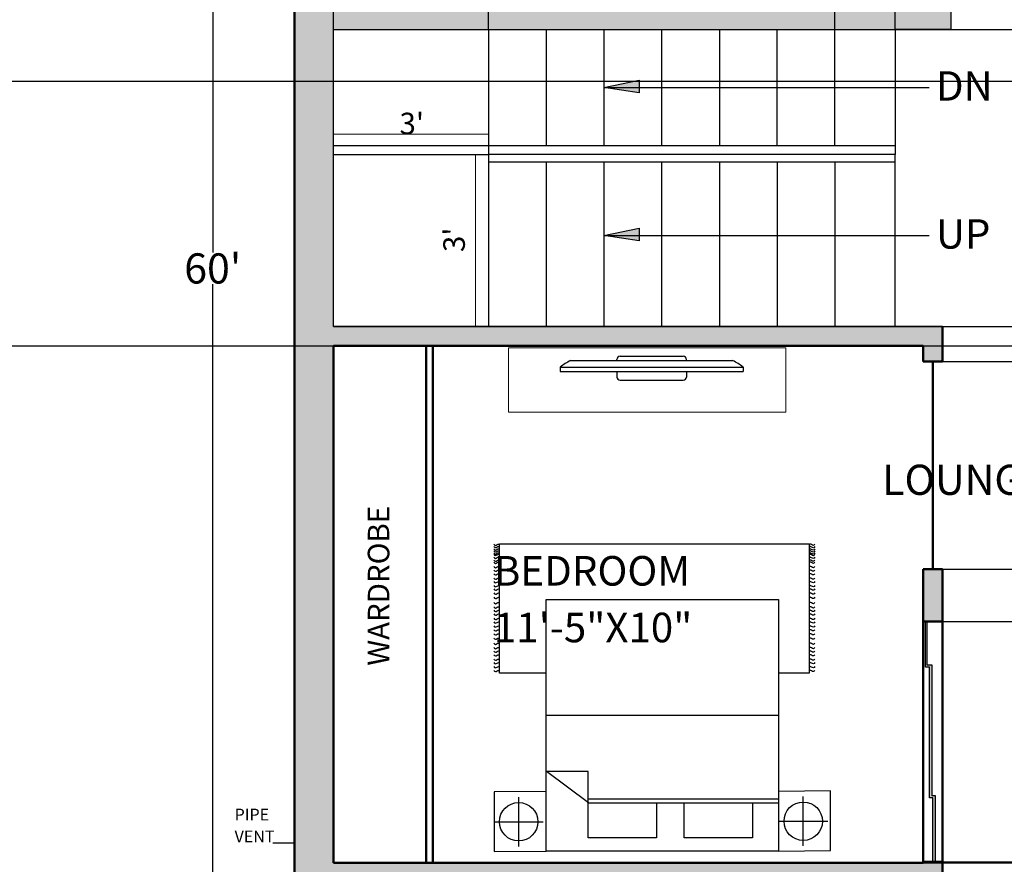
# Model space of a CAD drawing. Units: inches. Extents: x 48 to 822, y -191 to 651.
# Tile 9 of 13: x 445 to 673, y 101 to 297. Entities that reach past the tile are written whole.
import ezdxf

# ---------------------------------------------------------------- set-up
doc = ezdxf.new("R2010")
doc.units = ezdxf.units.IN
doc.header["$MEASUREMENT"] = 0
doc.layers.get('0').update_dxf_attribs({"color": 254})
for name, color, linetype, lineweight in [('A-ANNO-DIMS', 2, 'Continuous', 18), ('A-ANNO-TEXT', 3, 'Continuous', 25), ('A-AREA-IDEN', 7, 'Continuous', 25), ('A-FLOR-STRS', 3, 'Continuous', 25), ('A-FURN', 8, 'Continuous', 18), ('A-GLAZ', 4, 'Continuous', 25), ('A-WALL', 7, 'Continuous', 50), ('A-WALL-PATT', 8, 'Continuous', 13)]:
    doc.layers.add(name, color=color, linetype=linetype, lineweight=lineweight)
doc.layers.add('furniture', color=250, linetype='Continuous')
doc.styles.get("Standard").update_dxf_attribs({"font": 'arial.ttf'})
doc.dimstyles.get("Standard").update_dxf_attribs({"dimtxt": 7, "dimasz": 0.18, "dimexe": 0.18, "dimexo": 0.0625, "dimgap": 0.09, "dimtad": 0, "dimtih": 1, "dimtoh": 1, "dimzin": 0, "dimdsep": 46, "dimlunit": 3, "dimtxsty": 'Standard', "dimcen": 0.09, "dimadec": 0, "dimazin": 0, "dimtfac": 1, "dimtofl": 0, "dimtmove": 0, "dimatfit": 3, "dimfxl": 1, "dimtolj": 1, "dimtzin": 0, "dimarcsym": 0})

# ---------------------------------------------------------------- blocks, each defined once
blk = doc.blocks.new('CARPET')
at = {"layer": 'furniture'}
for p, q in [((-51.53, -98.11), (-51.53, -55.12)), ((-51.53, -55.12), (-41.27, -55.12)), ((36, -55.12), (51.55, -55.12)), ((51.55, -55.12), (51.55, -98.11)), ((51.55, -98.11), (-51.53, -98.11))]:
    blk.add_line(p, q, dxfattribs=at)
for points, knots in [([(-53.37, -55.99), (-53.22, -55.8), (-52.9, -55.41), (-52.34, -55.8), (-51.89, -56.08), (-51.65, -55.91), (-51.53, -55.83)], [0, 0, 0, 0, 0.653278, 1.290138, 1.740457, 2.114451, 2.114451, 2.114451, 2.114451]), ([(53.37, -55.99), (53.22, -55.8), (52.9, -55.41), (52.34, -55.8), (51.89, -56.08), (51.65, -55.91), (51.53, -55.83)], [0, 0, 0, 0, 0.653278, 1.290138, 1.740457, 2.114451, 2.114451, 2.114451, 2.114451]), ([(-53.37, -57.26), (-53.22, -57.07), (-52.9, -56.67), (-52.34, -57.07), (-51.89, -57.35), (-51.65, -57.17), (-51.53, -57.1)], [0, 0, 0, 0, 0.653278, 1.290138, 1.740457, 2.114451, 2.114451, 2.114451, 2.114451]), ([(-53.37, -58.59), (-53.22, -58.4), (-52.9, -58.01), (-52.34, -58.4), (-51.89, -58.68), (-51.65, -58.5), (-51.53, -58.43)], [0, 0, 0, 0, 0.653278, 1.290138, 1.740457, 2.114451, 2.114451, 2.114451, 2.114451]), ([(53.37, -57.26), (53.22, -57.07), (52.9, -56.67), (52.34, -57.07), (51.89, -57.35), (51.65, -57.17), (51.53, -57.1)], [0, 0, 0, 0, 0.653278, 1.290138, 1.740457, 2.114451, 2.114451, 2.114451, 2.114451]), ([(53.37, -58.59), (53.22, -58.4), (52.9, -58.01), (52.34, -58.4), (51.89, -58.68), (51.65, -58.5), (51.53, -58.43)], [0, 0, 0, 0, 0.653278, 1.290138, 1.740457, 2.114451, 2.114451, 2.114451, 2.114451]), ([(-53.37, -59.78), (-53.22, -59.58), (-52.9, -59.19), (-52.34, -59.58), (-51.89, -59.86), (-51.65, -59.69), (-51.53, -59.61)], [0, 0, 0, 0, 0.653278, 1.290138, 1.740457, 2.114451, 2.114451, 2.114451, 2.114451]), ([(-53.37, -61.22), (-53.22, -61.02), (-52.9, -60.63), (-52.34, -61.02), (-51.89, -61.3), (-51.65, -61.13), (-51.53, -61.05)], [0, 0, 0, 0, 0.653278, 1.290138, 1.740457, 2.114451, 2.114451, 2.114451, 2.114451]), ([(-53.37, -62.44), (-53.22, -62.25), (-52.9, -61.86), (-52.34, -62.25), (-51.89, -62.53), (-51.65, -62.36), (-51.53, -62.28)], [0, 0, 0, 0, 0.653278, 1.290138, 1.740457, 2.114451, 2.114451, 2.114451, 2.114451]), ([(53.37, -59.78), (53.22, -59.58), (52.9, -59.19), (52.34, -59.58), (51.89, -59.86), (51.65, -59.69), (51.53, -59.61)], [0, 0, 0, 0, 0.653278, 1.290138, 1.740457, 2.114451, 2.114451, 2.114451, 2.114451]), ([(53.37, -61.22), (53.22, -61.02), (52.9, -60.63), (52.34, -61.02), (51.89, -61.3), (51.65, -61.13), (51.53, -61.05)], [0, 0, 0, 0, 0.653278, 1.290138, 1.740457, 2.114451, 2.114451, 2.114451, 2.114451]), ([(53.37, -62.44), (53.22, -62.25), (52.9, -61.86), (52.34, -62.25), (51.89, -62.53), (51.65, -62.36), (51.53, -62.28)], [0, 0, 0, 0, 0.653278, 1.290138, 1.740457, 2.114451, 2.114451, 2.114451, 2.114451]), ([(-53.37, -63.63), (-53.22, -63.43), (-52.9, -63.04), (-52.34, -63.43), (-51.89, -63.72), (-51.65, -63.54), (-51.53, -63.46)], [0, 0, 0, 0, 0.653278, 1.290138, 1.740457, 2.114451, 2.114451, 2.114451, 2.114451]), ([(-53.37, -65.07), (-53.22, -64.87), (-52.9, -64.48), (-52.34, -64.87), (-51.89, -65.15), (-51.65, -64.98), (-51.53, -64.9)], [0, 0, 0, 0, 0.653278, 1.290138, 1.740457, 2.114451, 2.114451, 2.114451, 2.114451]), ([(53.37, -63.63), (53.22, -63.43), (52.9, -63.04), (52.34, -63.43), (51.89, -63.72), (51.65, -63.54), (51.53, -63.46)], [0, 0, 0, 0, 0.653278, 1.290138, 1.740457, 2.114451, 2.114451, 2.114451, 2.114451]), ([(53.37, -65.07), (53.22, -64.87), (52.9, -64.48), (52.34, -64.87), (51.89, -65.15), (51.65, -64.98), (51.53, -64.9)], [0, 0, 0, 0, 0.653278, 1.290138, 1.740457, 2.114451, 2.114451, 2.114451, 2.114451]), ([(-53.37, -66.76), (-53.22, -66.56), (-52.9, -66.17), (-52.34, -66.56), (-51.89, -66.84), (-51.65, -66.67), (-51.53, -66.59)], [0, 0, 0, 0, 0.653278, 1.290138, 1.740457, 2.114451, 2.114451, 2.114451, 2.114451]), ([(-53.37, -68.2), (-53.22, -68), (-52.9, -67.61), (-52.34, -68), (-51.89, -68.28), (-51.65, -68.11), (-51.53, -68.03)], [0, 0, 0, 0, 0.653278, 1.290138, 1.740457, 2.114451, 2.114451, 2.114451, 2.114451]), ([(53.37, -66.76), (53.22, -66.56), (52.9, -66.17), (52.34, -66.56), (51.89, -66.84), (51.65, -66.67), (51.53, -66.59)], [0, 0, 0, 0, 0.653278, 1.290138, 1.740457, 2.114451, 2.114451, 2.114451, 2.114451]), ([(53.37, -68.2), (53.22, -68), (52.9, -67.61), (52.34, -68), (51.89, -68.28), (51.65, -68.11), (51.53, -68.03)], [0, 0, 0, 0, 0.653278, 1.290138, 1.740457, 2.114451, 2.114451, 2.114451, 2.114451]), ([(-53.37, -69.53), (-53.22, -69.33), (-52.9, -68.94), (-52.34, -69.33), (-51.89, -69.61), (-51.65, -69.44), (-51.53, -69.36)], [0, 0, 0, 0, 0.653278, 1.290138, 1.740457, 2.114451, 2.114451, 2.114451, 2.114451]), ([(-53.37, -70.79), (-53.22, -70.6), (-52.9, -70.21), (-52.34, -70.6), (-51.89, -70.88), (-51.65, -70.7), (-51.53, -70.63)], [0, 0, 0, 0, 0.653278, 1.290138, 1.740457, 2.114451, 2.114451, 2.114451, 2.114451]), ([(-53.37, -72.12), (-53.22, -71.93), (-52.9, -71.54), (-52.34, -71.93), (-51.89, -72.21), (-51.65, -72.04), (-51.53, -71.96)], [0, 0, 0, 0, 0.653278, 1.290138, 1.740457, 2.114451, 2.114451, 2.114451, 2.114451]), ([(53.37, -69.53), (53.22, -69.33), (52.9, -68.94), (52.34, -69.33), (51.89, -69.61), (51.65, -69.44), (51.53, -69.36)], [0, 0, 0, 0, 0.653278, 1.290138, 1.740457, 2.114451, 2.114451, 2.114451, 2.114451]), ([(53.37, -70.79), (53.22, -70.6), (52.9, -70.21), (52.34, -70.6), (51.89, -70.88), (51.65, -70.7), (51.53, -70.63)], [0, 0, 0, 0, 0.653278, 1.290138, 1.740457, 2.114451, 2.114451, 2.114451, 2.114451]), ([(53.37, -72.12), (53.22, -71.93), (52.9, -71.54), (52.34, -71.93), (51.89, -72.21), (51.65, -72.04), (51.53, -71.96)], [0, 0, 0, 0, 0.653278, 1.290138, 1.740457, 2.114451, 2.114451, 2.114451, 2.114451]), ([(-53.37, -73.31), (-53.22, -73.11), (-52.9, -72.72), (-52.34, -73.11), (-51.89, -73.4), (-51.65, -73.22), (-51.53, -73.14)], [0, 0, 0, 0, 0.653278, 1.290138, 1.740457, 2.114451, 2.114451, 2.114451, 2.114451]), ([(-53.37, -74.75), (-53.22, -74.55), (-52.9, -74.16), (-52.34, -74.55), (-51.89, -74.83), (-51.65, -74.66), (-51.53, -74.58)], [0, 0, 0, 0, 0.653278, 1.290138, 1.740457, 2.114451, 2.114451, 2.114451, 2.114451]), ([(53.37, -73.31), (53.22, -73.11), (52.9, -72.72), (52.34, -73.11), (51.89, -73.4), (51.65, -73.22), (51.53, -73.14)], [0, 0, 0, 0, 0.653278, 1.290138, 1.740457, 2.114451, 2.114451, 2.114451, 2.114451]), ([(53.37, -74.75), (53.22, -74.55), (52.9, -74.16), (52.34, -74.55), (51.89, -74.83), (51.65, -74.66), (51.53, -74.58)], [0, 0, 0, 0, 0.653278, 1.290138, 1.740457, 2.114451, 2.114451, 2.114451, 2.114451]), ([(-53.37, -75.98), (-53.22, -75.78), (-52.9, -75.39), (-52.34, -75.78), (-51.89, -76.06), (-51.65, -75.89), (-51.53, -75.81)], [0, 0, 0, 0, 0.653278, 1.290138, 1.740457, 2.114451, 2.114451, 2.114451, 2.114451]), ([(-53.37, -77.16), (-53.22, -76.96), (-52.9, -76.57), (-52.34, -76.96), (-51.89, -77.25), (-51.65, -77.07), (-51.53, -76.99)], [0, 0, 0, 0, 0.653278, 1.290138, 1.740457, 2.114451, 2.114451, 2.114451, 2.114451]), ([(-53.37, -78.6), (-53.22, -78.4), (-52.9, -78.01), (-52.34, -78.4), (-51.89, -78.68), (-51.65, -78.51), (-51.53, -78.43)], [0, 0, 0, 0, 0.653278, 1.290138, 1.740457, 2.114451, 2.114451, 2.114451, 2.114451]), ([(53.37, -75.98), (53.22, -75.78), (52.9, -75.39), (52.34, -75.78), (51.89, -76.06), (51.65, -75.89), (51.53, -75.81)], [0, 0, 0, 0, 0.653278, 1.290138, 1.740457, 2.114451, 2.114451, 2.114451, 2.114451]), ([(53.37, -77.16), (53.22, -76.96), (52.9, -76.57), (52.34, -76.96), (51.89, -77.25), (51.65, -77.07), (51.53, -76.99)], [0, 0, 0, 0, 0.653278, 1.290138, 1.740457, 2.114451, 2.114451, 2.114451, 2.114451]), ([(53.37, -78.6), (53.22, -78.4), (52.9, -78.01), (52.34, -78.4), (51.89, -78.68), (51.65, -78.51), (51.53, -78.43)], [0, 0, 0, 0, 0.653278, 1.290138, 1.740457, 2.114451, 2.114451, 2.114451, 2.114451]), ([(-53.37, -80.29), (-53.22, -80.09), (-52.9, -79.7), (-52.34, -80.09), (-51.89, -80.37), (-51.65, -80.2), (-51.53, -80.12)], [0, 0, 0, 0, 0.653278, 1.290138, 1.740457, 2.114451, 2.114451, 2.114451, 2.114451]), ([(-53.37, -81.73), (-53.22, -81.53), (-52.9, -81.14), (-52.34, -81.53), (-51.89, -81.81), (-51.65, -81.64), (-51.53, -81.56)], [0, 0, 0, 0, 0.653278, 1.290138, 1.740457, 2.114451, 2.114451, 2.114451, 2.114451]), ([(53.37, -80.29), (53.22, -80.09), (52.9, -79.7), (52.34, -80.09), (51.89, -80.37), (51.65, -80.2), (51.53, -80.12)], [0, 0, 0, 0, 0.653278, 1.290138, 1.740457, 2.114451, 2.114451, 2.114451, 2.114451]), ([(53.37, -81.73), (53.22, -81.53), (52.9, -81.14), (52.34, -81.53), (51.89, -81.81), (51.65, -81.64), (51.53, -81.56)], [0, 0, 0, 0, 0.653278, 1.290138, 1.740457, 2.114451, 2.114451, 2.114451, 2.114451]), ([(-53.37, -83.06), (-53.22, -82.86), (-52.9, -82.47), (-52.34, -82.86), (-51.89, -83.14), (-51.65, -82.97), (-51.53, -82.89)], [0, 0, 0, 0, 0.653278, 1.290138, 1.740457, 2.114451, 2.114451, 2.114451, 2.114451]), ([(-53.37, -84.18), (-53.22, -83.99), (-52.9, -83.6), (-52.34, -83.99), (-51.89, -84.27), (-51.65, -84.09), (-51.53, -84.02)], [0, 0, 0, 0, 0.653278, 1.290138, 1.740457, 2.114451, 2.114451, 2.114451, 2.114451]), ([(-53.37, -85.51), (-53.22, -85.32), (-52.9, -84.93), (-52.34, -85.32), (-51.89, -85.6), (-51.65, -85.42), (-51.53, -85.35)], [0, 0, 0, 0, 0.653278, 1.290138, 1.740457, 2.114451, 2.114451, 2.114451, 2.114451]), ([(53.37, -83.06), (53.22, -82.86), (52.9, -82.47), (52.34, -82.86), (51.89, -83.14), (51.65, -82.97), (51.53, -82.89)], [0, 0, 0, 0, 0.653278, 1.290138, 1.740457, 2.114451, 2.114451, 2.114451, 2.114451]), ([(53.37, -84.18), (53.22, -83.99), (52.9, -83.6), (52.34, -83.99), (51.89, -84.27), (51.65, -84.09), (51.53, -84.02)], [0, 0, 0, 0, 0.653278, 1.290138, 1.740457, 2.114451, 2.114451, 2.114451, 2.114451]), ([(53.37, -85.51), (53.22, -85.32), (52.9, -84.93), (52.34, -85.32), (51.89, -85.6), (51.65, -85.42), (51.53, -85.35)], [0, 0, 0, 0, 0.653278, 1.290138, 1.740457, 2.114451, 2.114451, 2.114451, 2.114451]), ([(-53.37, -86.7), (-53.22, -86.5), (-52.9, -86.11), (-52.34, -86.5), (-51.89, -86.78), (-51.65, -86.61), (-51.53, -86.53)], [0, 0, 0, 0, 0.653278, 1.290138, 1.740457, 2.114451, 2.114451, 2.114451, 2.114451]), ([(-53.37, -88.14), (-53.22, -87.94), (-52.9, -87.55), (-52.34, -87.94), (-51.89, -88.22), (-51.65, -88.05), (-51.53, -87.97)], [0, 0, 0, 0, 0.653278, 1.290138, 1.740457, 2.114451, 2.114451, 2.114451, 2.114451]), ([(53.37, -86.7), (53.22, -86.5), (52.9, -86.11), (52.34, -86.5), (51.89, -86.78), (51.65, -86.61), (51.53, -86.53)], [0, 0, 0, 0, 0.653278, 1.290138, 1.740457, 2.114451, 2.114451, 2.114451, 2.114451]), ([(53.37, -88.14), (53.22, -87.94), (52.9, -87.55), (52.34, -87.94), (51.89, -88.22), (51.65, -88.05), (51.53, -87.97)], [0, 0, 0, 0, 0.653278, 1.290138, 1.740457, 2.114451, 2.114451, 2.114451, 2.114451]), ([(-53.37, -89.36), (-53.22, -89.17), (-52.9, -88.78), (-52.34, -89.17), (-51.89, -89.45), (-51.65, -89.28), (-51.53, -89.2)], [0, 0, 0, 0, 0.653278, 1.290138, 1.740457, 2.114451, 2.114451, 2.114451, 2.114451]), ([(-53.37, -90.55), (-53.22, -90.35), (-52.9, -89.96), (-52.34, -90.35), (-51.89, -90.64), (-51.65, -90.46), (-51.53, -90.38)], [0, 0, 0, 0, 0.653278, 1.290138, 1.740457, 2.114451, 2.114451, 2.114451, 2.114451]), ([(-53.37, -91.99), (-53.22, -91.79), (-52.9, -91.4), (-52.34, -91.79), (-51.89, -92.07), (-51.65, -91.9), (-51.53, -91.82)], [0, 0, 0, 0, 0.653278, 1.290138, 1.740457, 2.114451, 2.114451, 2.114451, 2.114451]), ([(53.37, -89.36), (53.22, -89.17), (52.9, -88.78), (52.34, -89.17), (51.89, -89.45), (51.65, -89.28), (51.53, -89.2)], [0, 0, 0, 0, 0.653278, 1.290138, 1.740457, 2.114451, 2.114451, 2.114451, 2.114451]), ([(53.37, -90.55), (53.22, -90.35), (52.9, -89.96), (52.34, -90.35), (51.9, -90.63), (51.66, -90.47), (51.55, -90.4)], [0, 0, 0, 0, 0.653278, 1.290138, 1.740457, 2.0926, 2.0926, 2.0926, 2.0926]), ([(53.37, -91.99), (53.22, -91.79), (52.9, -91.4), (52.34, -91.79), (51.9, -92.07), (51.66, -91.91), (51.55, -91.83)], [0, 0, 0, 0, 0.653278, 1.290138, 1.740457, 2.0926, 2.0926, 2.0926, 2.0926]), ([(-53.37, -92.69), (-53.22, -92.48), (-52.9, -92.08), (-52.35, -92.49), (-51.89, -92.77), (-51.65, -92.6), (-51.53, -92.52)], [0, 0, 0, 0, 0.663904, 1.307406, 1.757725, 2.131719, 2.131719, 2.131719, 2.131719]), ([(-53.37, -93.61), (-53.22, -93.42), (-52.9, -93.03), (-52.34, -93.42), (-51.89, -93.7), (-51.65, -93.52), (-51.53, -93.45)], [0, 0, 0, 0, 0.653278, 1.290138, 1.740457, 2.114451, 2.114451, 2.114451, 2.114451]), ([(-53.37, -94.55), (-53.22, -94.35), (-52.9, -93.96), (-52.34, -94.35), (-51.89, -94.63), (-51.65, -94.46), (-51.53, -94.38)], [0, 0, 0, 0, 0.653278, 1.290138, 1.740457, 2.114451, 2.114451, 2.114451, 2.114451]), ([(-53.37, -95.05), (-53.22, -94.85), (-52.9, -94.46), (-52.34, -94.85), (-51.89, -95.14), (-51.65, -94.96), (-51.53, -94.88)], [0, 0, 0, 0, 0.653278, 1.290138, 1.740457, 2.114451, 2.114451, 2.114451, 2.114451]), ([(53.37, -92.69), (53.22, -92.49), (52.9, -92.09), (52.34, -92.49), (51.9, -92.77), (51.66, -92.61), (51.55, -92.53)], [0, 0, 0, 0, 0.656792, 1.295826, 1.746145, 2.098292, 2.098292, 2.098292, 2.098292]), ([(53.37, -93.66), (53.22, -93.46), (52.9, -93.07), (52.34, -93.46), (51.9, -93.74), (51.66, -93.58), (51.55, -93.5)], [0, 0, 0, 0, 0.653278, 1.290138, 1.740457, 2.0926, 2.0926, 2.0926, 2.0926]), ([(53.37, -94.59), (53.22, -94.4), (52.9, -94.01), (52.34, -94.4), (51.9, -94.68), (51.66, -94.51), (51.55, -94.44)], [0, 0, 0, 0, 0.653278, 1.290138, 1.740457, 2.0926, 2.0926, 2.0926, 2.0926]), ([(53.37, -95.1), (53.22, -94.9), (52.9, -94.51), (52.34, -94.9), (51.9, -95.18), (51.66, -95.02), (51.55, -94.94)], [0, 0, 0, 0, 0.653278, 1.290138, 1.740457, 2.0926, 2.0926, 2.0926, 2.0926]), ([(-53.37, -95.73), (-53.22, -95.54), (-52.9, -95.15), (-52.34, -95.54), (-51.89, -95.82), (-51.65, -95.65), (-51.53, -95.57)], [0, 0, 0, 0, 0.653278, 1.290138, 1.740457, 2.114451, 2.114451, 2.114451, 2.114451]), ([(-53.37, -96.38), (-53.22, -96.18), (-52.9, -95.79), (-52.34, -96.18), (-51.89, -96.47), (-51.65, -96.29), (-51.53, -96.21)], [0, 0, 0, 0, 0.653278, 1.290138, 1.740457, 2.114451, 2.114451, 2.114451, 2.114451]), ([(-53.37, -97.17), (-53.22, -96.98), (-52.9, -96.59), (-52.34, -96.98), (-51.89, -97.26), (-51.65, -97.08), (-51.53, -97.01)], [0, 0, 0, 0, 0.653278, 1.290138, 1.740457, 2.114451, 2.114451, 2.114451, 2.114451]), ([(-53.37, -97.99), (-53.22, -97.79), (-52.9, -97.4), (-52.34, -97.79), (-51.89, -98.08), (-51.65, -97.9), (-51.53, -97.82)], [0, 0, 0, 0, 0.653278, 1.290138, 1.740457, 2.114451, 2.114451, 2.114451, 2.114451]), ([(53.37, -95.78), (53.22, -95.58), (52.9, -95.19), (52.34, -95.58), (51.89, -95.86), (51.65, -95.69), (51.53, -95.61)], [0, 0, 0, 0, 0.653278, 1.290138, 1.740457, 2.114451, 2.114451, 2.114451, 2.114451]), ([(53.37, -96.43), (53.22, -96.23), (52.9, -95.84), (52.34, -96.23), (51.89, -96.51), (51.65, -96.34), (51.53, -96.26)], [0, 0, 0, 0, 0.653278, 1.290138, 1.740457, 2.114451, 2.114451, 2.114451, 2.114451]), ([(53.37, -97.22), (53.22, -97.02), (52.9, -96.63), (52.34, -97.02), (51.89, -97.3), (51.65, -97.13), (51.53, -97.05)], [0, 0, 0, 0, 0.653278, 1.290138, 1.740457, 2.114451, 2.114451, 2.114451, 2.114451]), ([(53.37, -97.99), (53.22, -97.79), (52.9, -97.4), (52.34, -97.79), (51.89, -98.08), (51.65, -97.9), (51.53, -97.82)], [0, 0, 0, 0, 0.653278, 1.290138, 1.740457, 2.114451, 2.114451, 2.114451, 2.114451])]:
    blk.add_open_spline(points, degree=3, knots=knots, dxfattribs=at)
blk = doc.blocks.new('A$C58D270C6')
at = {"layer": 'furniture'}
for p, q in [((9.09, 124.13), (9.09, 108.87)), ((1.46, 116.5), (16.73, 116.5)), ((14.97, 94.84), (24.62, 107.92)), ((24.62, 94.93), (24.62, 107.92)), ((42.08, 108), (42.08, 36)), ((14.97, 94.93), (24.62, 94.93)), ((14.97, 94.84), (14.97, 36)), ((16.22, 94.93), (16.22, 36)), ((9.25, 36), (9.25, 20.74)), ((1.62, 28.37), (16.88, 28.37))]:
    blk.add_line(p, q, dxfattribs=at)
for points in [[(18.5, 108), (18.34, 124.13), (-0.16, 124.13), (0, 108)], [(0, 108), (77.91, 108), (77.91, 36), (0, 36)], [(4.09, 94.93), (14.97, 94.93), (14.97, 73.83), (4.09, 73.83)], [(4.09, 65.23), (14.97, 65.23), (14.97, 44.13), (4.09, 44.13)], [(18.65, 19.87), (18.5, 36), (0, 36), (0.16, 19.87)]]:
    blk.add_lwpolyline(points, close=True, dxfattribs=at)
for centre in [(9.09, 116.5), (9.25, 28.37)]:
    blk.add_circle(centre, 5.95, dxfattribs=at)
at = {"layer": 'furniture', "xscale": 0.9312884925094044, "yscale": 0.9312884925094044, "zscale": 0.9312884925094044, "rotation": 90}
blk.add_blockref('CARPET', (3.79, 74.47), dxfattribs=at)
blk = doc.blocks.new('PLASMA-LARGE')
at = {"layer": 'furniture'}
for p, q in [((-7.26, 0), (7.26, 0)), ((-18.61, -1), (18.61, -1)), ((-8, -1), (-8, -0.74)), ((8, -1), (8, -0.74)), ((-21, -2.5), (21, -2.5)), ((-21, -2.5), (-21, -3.5)), ((-21, -3.5), (21, -3.5)), ((-8, -3.5), (-8, -4.76)), ((8, -3.5), (8, -4.76)), ((21, -2.5), (21, -3.5)), ((-7.26, -5.5), (7.26, -5.5))]:
    blk.add_line(p, q, dxfattribs=at)
for centre, radius, start, end in [((-7.26, -0.74), 0.744, 90, 180), ((7.26, -0.74), 0.744, 0, 90), ((-13.97, -11.05), 11.07, 114.7602, 129.4175), ((13.97, -11.05), 11.07, 50.5825, 65.2398), ((-7.26, -4.76), 0.744, 180, 270), ((7.26, -4.76), 0.744, 270, 0)]:
    blk.add_arc(centre, radius, start, end, dxfattribs=at)
blk = doc.blocks.new('*D19')
at = {"layer": 'A-ANNO-DIMS', "color": 0, "lineweight": -2, "transparency": 16777216}
for p, q in [((489.56, 599.69), (489.41, 599.69)), ((489.59, 599.51), (489.59, 243.35)), ((489.59, -120.13), (489.59, 236.02)), ((489.56, -120.31), (489.41, -120.31))]:
    blk.add_line(p, q, dxfattribs=at)
at = {"layer": 'A-ANNO-DIMS', "color": 0, "transparency": 16777216}
for points in [[(489.56, 599.51), (489.62, 599.51), (489.59, 599.69)], [(489.56, -120.13), (489.62, -120.13), (489.59, -120.31)]]:
    blk.add_solid(points, dxfattribs=at)
at = {"layer": 'Defpoints', "color": 0, "transparency": 16777216}
for p in [(489.62, 599.69), (489.59, -120.31), (489.62, -120.31)]:
    blk.add_point(p, dxfattribs=at)
at = {"layer": 'A-ANNO-DIMS', "color": 0, "transparency": 16777216, "insert": (489.59, 239.69), "char_height": 7, "attachment_point": 5}
blk.add_mtext("\\A1;60'", dxfattribs=at)
blk = doc.blocks.new('WIN-1500')
for p, q in [((315.51, 546.44), (315.51, 547.24)), ((315.51, 547.24), (345.84, 547.24)), ((345.84, 547.24), (345.84, 548.17)), ((345.84, 548.17), (356.45, 548.17)), ((346.31, 546.59), (346.31, 547.73)), ((346.31, 547.73), (356.45, 547.73)), ((300.62, 546.44), (315.51, 546.44)), ((300.62, 545.8), (315.95, 545.8)), ((315.95, 545.8), (315.95, 546.59)), ((315.95, 546.59), (346.31, 546.59))]:
    blk.add_line(p, q)
blk = doc.blocks.new('TV-UNIT')
for p, q in [((14.9, 64.44), (0, 64.44)), ((0, 64.44), (0, 0)), ((14.9, 64.44), (14.9, 0)), ((0, 0), (14.9, 0))]:
    blk.add_line(p, q)
blk = doc.blocks.new('STAIR-ARROW')
for p, q in [((0, 1.28), (8.17, 2.92)), ((8.17, 2.92), (8.17, 0)), ((0, 1.28), (75.57, 1.28)), ((8.17, 0), (0, 1.28))]:
    blk.add_line(p, q)
blk = doc.blocks.new('*D52')
at = {"layer": 'A-ANNO-DIMS', "color": 0, "lineweight": -2, "transparency": 16777216}
for p, q in [((713, 201.45), (709.64, 201.45)), ((709.82, 201.27), (709.82, 194.33)), ((709.82, 179.96), (709.82, 186.9)), ((713, 179.78), (709.64, 179.78))]:
    blk.add_line(p, q, dxfattribs=at)
at = {"layer": 'A-ANNO-DIMS', "color": 0, "transparency": 16777216}
for points in [[(709.79, 201.27), (709.85, 201.27), (709.82, 201.45)], [(709.79, 179.96), (709.85, 179.96), (709.82, 179.78)]]:
    blk.add_solid(points, dxfattribs=at)
at = {"layer": 'Defpoints', "color": 0, "transparency": 16777216}
for p in [(709.82, 201.45), (713.07, 201.45), (713.07, 179.78)]:
    blk.add_point(p, dxfattribs=at)
at = {"layer": 'A-ANNO-DIMS', "color": 0, "transparency": 16777216, "insert": (709.82, 190.62), "char_height": 7, "attachment_point": 5}
blk.add_mtext('\\A1;LOUNGE CHAIR 1\'-9 1/2" TYP.', dxfattribs=at)
blk = doc.blocks.new('*D85')
at = {"layer": 'A-ANNO-DIMS', "color": 0, "lineweight": -2, "transparency": 16777216}
for p, q in [((321.36, 283.18), (790.04, 283.18)), ((789.86, 283), (789.86, 256.14)), ((789.86, 221.87), (789.86, 248.73)), ((321.2, 221.69), (790.04, 221.69))]:
    blk.add_line(p, q, dxfattribs=at)
at = {"layer": 'A-ANNO-DIMS', "color": 0, "transparency": 16777216}
for points in [[(789.83, 283), (789.89, 283), (789.86, 283.18)], [(789.83, 221.87), (789.89, 221.87), (789.86, 221.69)]]:
    blk.add_solid(points, dxfattribs=at)
at = {"layer": 'Defpoints', "color": 0, "transparency": 16777216}
for p in [(321.3, 283.18), (321.14, 221.69), (789.86, 221.69)]:
    blk.add_point(p, dxfattribs=at)
at = {"layer": 'A-ANNO-DIMS', "color": 0, "transparency": 16777216, "insert": (789.86, 252.44), "char_height": 7, "attachment_point": 5}
blk.add_mtext('\\A1;5\'-1 1/2"', dxfattribs=at)
blk = doc.blocks.new('*D110')
at = {"layer": 'A-ANNO-DIMS', "color": 0, "lineweight": -2, "transparency": 16777216}
for p, q in [((517.67, 299.69), (790.04, 299.69)), ((789.86, 299.51), (789.86, 295.37)), ((517.67, 295.19), (790.04, 295.19)), ((789.86, 295.19), (789.86, 295.01)), ((789.86, 295.01), (789.68, 295.01))]:
    blk.add_line(p, q, dxfattribs=at)
at = {"layer": 'A-ANNO-DIMS', "color": 0, "transparency": 16777216}
for points in [[(789.83, 299.51), (789.89, 299.51), (789.86, 299.69)], [(789.83, 295.37), (789.89, 295.37), (789.86, 295.19)]]:
    blk.add_solid(points, dxfattribs=at)
at = {"layer": 'Defpoints', "color": 0, "transparency": 16777216}
for p in [(517.61, 299.69), (517.61, 295.19), (789.86, 295.19)]:
    blk.add_point(p, dxfattribs=at)
at = {"layer": 'A-ANNO-DIMS', "color": 0, "transparency": 16777216, "insert": (772.13, 295.01), "char_height": 7, "attachment_point": 5}
blk.add_mtext('\\A1;0\'-4 1/2"', dxfattribs=at)
blk = doc.blocks.new('*D111')
at = {"layer": 'A-ANNO-DIMS', "color": 0, "lineweight": -2, "transparency": 16777216}
for p, q in [((517.67, 295.19), (790.04, 295.19)), ((789.86, 295.01), (789.86, 264.35)), ((789.86, 226.37), (789.86, 257.02)), ((517.67, 226.19), (790.04, 226.19))]:
    blk.add_line(p, q, dxfattribs=at)
at = {"layer": 'A-ANNO-DIMS', "color": 0, "transparency": 16777216}
for points in [[(789.83, 295.01), (789.89, 295.01), (789.86, 295.19)], [(789.83, 226.37), (789.89, 226.37), (789.86, 226.19)]]:
    blk.add_solid(points, dxfattribs=at)
at = {"layer": 'Defpoints', "color": 0, "transparency": 16777216}
for p in [(517.61, 295.19), (517.61, 226.19), (789.86, 226.19)]:
    blk.add_point(p, dxfattribs=at)
at = {"layer": 'A-ANNO-DIMS', "color": 0, "transparency": 16777216, "insert": (789.86, 260.69), "char_height": 7, "attachment_point": 5}
blk.add_mtext('\\A1;5\'-9"', dxfattribs=at)
blk = doc.blocks.new('*D112')
at = {"layer": 'A-ANNO-DIMS', "color": 0, "lineweight": -2, "transparency": 16777216}
for p, q in [((517.67, 226.19), (790.04, 226.19)), ((789.86, 226.01), (789.86, 221.87)), ((517.67, 221.69), (790.04, 221.69)), ((789.86, 221.51), (789.68, 221.51)), ((789.86, 221.69), (789.86, 221.51))]:
    blk.add_line(p, q, dxfattribs=at)
at = {"layer": 'A-ANNO-DIMS', "color": 0, "transparency": 16777216}
for points in [[(789.83, 226.01), (789.89, 226.01), (789.86, 226.19)], [(789.83, 221.87), (789.89, 221.87), (789.86, 221.69)]]:
    blk.add_solid(points, dxfattribs=at)
at = {"layer": 'Defpoints', "color": 0, "transparency": 16777216}
for p in [(517.61, 226.19), (517.61, 221.69), (789.86, 221.69)]:
    blk.add_point(p, dxfattribs=at)
at = {"layer": 'A-ANNO-DIMS', "color": 0, "transparency": 16777216, "insert": (772.13, 221.51), "char_height": 7, "attachment_point": 5}
blk.add_mtext('\\A1;0\'-4 1/2"', dxfattribs=at)
blk = doc.blocks.new('*D113')
at = {"layer": 'A-ANNO-DIMS', "color": 0, "lineweight": -2, "transparency": 16777216}
for p, q in [((517.67, 221.69), (790.04, 221.69)), ((789.86, 221.51), (789.86, 165.35)), ((789.86, 101.87), (789.86, 158.02)), ((517.67, 101.69), (790.04, 101.69))]:
    blk.add_line(p, q, dxfattribs=at)
at = {"layer": 'A-ANNO-DIMS', "color": 0, "transparency": 16777216}
for points in [[(789.83, 221.51), (789.89, 221.51), (789.86, 221.69)], [(789.83, 101.87), (789.89, 101.87), (789.86, 101.69)]]:
    blk.add_solid(points, dxfattribs=at)
at = {"layer": 'Defpoints', "color": 0, "transparency": 16777216}
for p in [(517.61, 221.69), (517.61, 101.69), (789.86, 101.69)]:
    blk.add_point(p, dxfattribs=at)
at = {"layer": 'A-ANNO-DIMS', "color": 0, "transparency": 16777216, "insert": (789.86, 161.69), "char_height": 7, "attachment_point": 5}
blk.add_mtext('\\A1;10\'-0"', dxfattribs=at)
blk = doc.blocks.new('*D114')
at = {"layer": 'A-ANNO-DIMS', "color": 0, "lineweight": -2, "transparency": 16777216}
for p, q in [((517.67, 101.69), (790.04, 101.69)), ((789.86, 101.51), (789.86, 97.37)), ((517.67, 97.19), (790.04, 97.19)), ((789.86, 97.01), (789.68, 97.01)), ((789.86, 97.19), (789.86, 97.01))]:
    blk.add_line(p, q, dxfattribs=at)
at = {"layer": 'A-ANNO-DIMS', "color": 0, "transparency": 16777216}
for points in [[(789.83, 101.51), (789.89, 101.51), (789.86, 101.69)], [(789.83, 97.37), (789.89, 97.37), (789.86, 97.19)]]:
    blk.add_solid(points, dxfattribs=at)
at = {"layer": 'Defpoints', "color": 0, "transparency": 16777216}
for p in [(517.61, 101.69), (517.61, 97.19), (789.86, 97.19)]:
    blk.add_point(p, dxfattribs=at)
at = {"layer": 'A-ANNO-DIMS', "color": 0, "transparency": 16777216, "insert": (772.13, 97.01), "char_height": 7, "attachment_point": 5}
blk.add_mtext('\\A1;0\'-4 1/2"', dxfattribs=at)
blk = doc.blocks.new('*D124')
at = {"layer": 'A-ANNO-DIMS', "color": 0, "lineweight": -2, "transparency": 16777216}
for p, q in [((517.61, 295.25), (517.61, 641.12)), ((517.79, 640.94), (526.22, 640.94)), ((553.43, 640.94), (545, 640.94)), ((553.61, 295.25), (553.61, 641.12))]:
    blk.add_line(p, q, dxfattribs=at)
at = {"layer": 'A-ANNO-DIMS', "color": 0, "transparency": 16777216}
for points in [[(517.79, 640.97), (517.79, 640.91), (517.61, 640.94)], [(553.43, 640.97), (553.43, 640.91), (553.61, 640.94)]]:
    blk.add_solid(points, dxfattribs=at)
at = {"layer": 'Defpoints', "color": 0, "transparency": 16777216}
for p in [(553.61, 640.94), (517.61, 295.19), (553.61, 295.19)]:
    blk.add_point(p, dxfattribs=at)
at = {"layer": 'A-ANNO-DIMS', "color": 0, "transparency": 16777216, "insert": (535.61, 640.94), "char_height": 7, "attachment_point": 5}
blk.add_mtext('\\A1;3\'-0"', dxfattribs=at)
blk = doc.blocks.new('*D125')
at = {"layer": 'A-ANNO-DIMS', "color": 0, "lineweight": -2, "transparency": 16777216}
for p, q in [((634.1, 295.25), (634.1, 641.12)), ((634.28, 640.94), (647.91, 640.94)), ((648.09, 295.25), (648.09, 641.12)), ((648.09, 640.94), (648.27, 640.94))]:
    blk.add_line(p, q, dxfattribs=at)
at = {"layer": 'A-ANNO-DIMS', "color": 0, "transparency": 16777216}
for points in [[(634.28, 640.97), (634.28, 640.91), (634.1, 640.94)], [(647.91, 640.97), (647.91, 640.91), (648.09, 640.94)]]:
    blk.add_solid(points, dxfattribs=at)
at = {"layer": 'Defpoints', "color": 0, "transparency": 16777216}
for p in [(648.09, 640.94), (634.1, 295.19), (648.09, 295.19)]:
    blk.add_point(p, dxfattribs=at)
at = {"layer": 'A-ANNO-DIMS', "color": 0, "transparency": 16777216, "insert": (657.33, 640.94), "char_height": 7, "attachment_point": 5}
blk.add_mtext('\\A1;1\'-2"', dxfattribs=at)
blk = doc.blocks.new('*D126')
at = {"layer": 'A-ANNO-DIMS', "color": 0, "lineweight": -2, "transparency": 16777216}
for p, q in [((553.61, 295.25), (553.61, 641.12)), ((553.79, 640.94), (580.61, 640.94)), ((647.91, 640.94), (621.09, 640.94)), ((648.09, 295.25), (648.09, 641.12))]:
    blk.add_line(p, q, dxfattribs=at)
at = {"layer": 'A-ANNO-DIMS', "color": 0, "transparency": 16777216}
for points in [[(553.79, 640.97), (553.79, 640.91), (553.61, 640.94)], [(647.91, 640.97), (647.91, 640.91), (648.09, 640.94)]]:
    blk.add_solid(points, dxfattribs=at)
at = {"layer": 'Defpoints', "color": 0, "transparency": 16777216}
for p in [(648.09, 640.94), (553.61, 295.19), (648.09, 295.19)]:
    blk.add_point(p, dxfattribs=at)
at = {"layer": 'A-ANNO-DIMS', "color": 0, "transparency": 16777216, "insert": (600.85, 640.94), "char_height": 7, "attachment_point": 5}
blk.add_mtext('\\A1;7\'-10 1/2"', dxfattribs=at)
blk = doc.blocks.new('*D127')
at = {"layer": 'A-ANNO-DIMS', "color": 0, "lineweight": -2, "transparency": 16777216}
for p, q in [((659.17, 218.07), (790.04, 218.07)), ((789.86, 217.89), (789.86, 197.63)), ((789.86, 170.05), (789.86, 190.31)), ((659.17, 169.87), (790.04, 169.87))]:
    blk.add_line(p, q, dxfattribs=at)
at = {"layer": 'A-ANNO-DIMS', "color": 0, "transparency": 16777216}
for points in [[(789.83, 217.89), (789.89, 217.89), (789.86, 218.07)], [(789.83, 170.05), (789.89, 170.05), (789.86, 169.87)]]:
    blk.add_solid(points, dxfattribs=at)
at = {"layer": 'Defpoints', "color": 0, "transparency": 16777216}
for p in [(659.11, 218.07), (659.11, 169.87), (789.86, 169.87)]:
    blk.add_point(p, dxfattribs=at)
at = {"layer": 'A-ANNO-DIMS', "color": 0, "transparency": 16777216, "insert": (789.86, 193.97), "char_height": 7, "attachment_point": 5}
blk.add_mtext('\\A1;4\'-0"', dxfattribs=at)
blk = doc.blocks.new('*D128')
at = {"layer": 'A-ANNO-DIMS', "color": 0, "lineweight": -2, "transparency": 16777216}
for p, q in [((659.17, 169.87), (790.04, 169.87)), ((789.86, 169.69), (789.86, 167.46)), ((789.86, 157.9), (789.86, 160.13)), ((659.17, 157.72), (790.04, 157.72))]:
    blk.add_line(p, q, dxfattribs=at)
at = {"layer": 'A-ANNO-DIMS', "color": 0, "transparency": 16777216}
for points in [[(789.83, 169.69), (789.89, 169.69), (789.86, 169.87)], [(789.83, 157.9), (789.89, 157.9), (789.86, 157.72)]]:
    blk.add_solid(points, dxfattribs=at)
at = {"layer": 'Defpoints', "color": 0, "transparency": 16777216}
for p in [(659.11, 169.87), (659.11, 157.72), (789.86, 157.72)]:
    blk.add_point(p, dxfattribs=at)
at = {"layer": 'A-ANNO-DIMS', "color": 0, "transparency": 16777216, "insert": (789.86, 163.8), "char_height": 7, "attachment_point": 5}
blk.add_mtext('\\A1;1\'-0"', dxfattribs=at)
blk = doc.blocks.new('*D129')
at = {"layer": 'A-ANNO-DIMS', "color": 0, "lineweight": -2, "transparency": 16777216}
for p, q in [((659.17, 157.72), (790.04, 157.72)), ((789.86, 157.54), (789.86, 133.47)), ((789.86, 102.08), (789.86, 126.14)), ((659.17, 101.9), (790.04, 101.9))]:
    blk.add_line(p, q, dxfattribs=at)
at = {"layer": 'A-ANNO-DIMS', "color": 0, "transparency": 16777216}
for points in [[(789.83, 157.54), (789.89, 157.54), (789.86, 157.72)], [(789.83, 102.08), (789.89, 102.08), (789.86, 101.9)]]:
    blk.add_solid(points, dxfattribs=at)
at = {"layer": 'Defpoints', "color": 0, "transparency": 16777216}
for p in [(659.11, 157.72), (659.11, 101.9), (789.86, 101.9)]:
    blk.add_point(p, dxfattribs=at)
at = {"layer": 'A-ANNO-DIMS', "color": 0, "transparency": 16777216, "insert": (789.86, 129.81), "char_height": 7, "attachment_point": 5}
blk.add_mtext('\\A1;4\'-8"', dxfattribs=at)
blk = doc.blocks.new('*D130')
at = {"layer": 'A-ANNO-DIMS', "color": 0, "lineweight": -2, "transparency": 16777216}
for p, q in [((659.17, 101.9), (790.04, 101.9)), ((789.86, 101.72), (789.86, 69.94)), ((789.86, 30.74), (789.86, 62.52)), ((659.17, 30.56), (790.04, 30.56))]:
    blk.add_line(p, q, dxfattribs=at)
at = {"layer": 'A-ANNO-DIMS', "color": 0, "transparency": 16777216}
for points in [[(789.83, 101.72), (789.89, 101.72), (789.86, 101.9)], [(789.83, 30.74), (789.89, 30.74), (789.86, 30.56)]]:
    blk.add_solid(points, dxfattribs=at)
at = {"layer": 'Defpoints', "color": 0, "transparency": 16777216}
for p in [(659.11, 101.9), (659.11, 30.56), (789.86, 30.56)]:
    blk.add_point(p, dxfattribs=at)
at = {"layer": 'A-ANNO-DIMS', "color": 0, "transparency": 16777216, "insert": (789.86, 66.23), "char_height": 7, "attachment_point": 5}
blk.add_mtext('\\A1;5\'-11 1/2"', dxfattribs=at)

msp = doc.modelspace()

# ---------------------------------------------------------------- hatches: boundary and pattern name
at = {"layer": 'A-FLOR-STRS'}
h = msp.add_hatch(color=256, dxfattribs=at)
h.dxf.hatch_style = 1
h.paths.add_polyline_path([(588.607, 283.366), (580.441, 281.722), (588.607, 280.445)])
h = msp.add_hatch(color=256, dxfattribs=at)
h.dxf.hatch_style = 1
h.paths.add_polyline_path([(588.607, 249.006), (580.441, 247.361), (588.607, 246.084)])
at = {"layer": 'A-WALL-PATT'}
h = msp.add_hatch(color=256, dxfattribs=at)
h.dxf.hatch_style = 1
h.paths.add_polyline_path([(614.11, 432.437), (609.61, 432.437), (609.61, 376.187), (535.284, 376.187), (535.284, 371.687), (547.61, 371.687), (547.61, 359.12), (552.11, 359.12), (552.11, 371.687), (609.61, 371.687), (609.61, 335.687), (614.11, 335.687)], flags=17)
h.paths.add_polyline_path([(614.11, 434.687), (609.61, 434.687), (609.61, 432.437), (614.11, 432.437)], flags=17)
h.paths.add_polyline_path([(573.934, 434.687), (517.61, 434.687), (517.61, 590.687), (650.61, 590.687), (650.61, 585.522), (655.11, 585.522), (655.11, 590.687), (739.61, 590.687), (739.61, 548.687), (655.11, 548.687), (655.11, 550.72), (650.61, 550.72), (650.61, 458.608), (655.11, 458.608), (655.11, 544.187), (739.61, 544.187), (739.61, 434.541), (650.61, 434.541), (650.61, 430.041), (739.61, 430.041), (739.61, -16.844), (729.973, -16.844), (729.973, -21.344), (748.61, -21.344), (748.61, 599.687), (508.61, 599.687), (508.61, -120.313), (543.114, -120.313), (543.114, -111.313), (517.61, -111.313), (517.61, 38.687), (607.29, 38.687), (607.29, 43.187), (517.61, 43.187), (517.61, 97.187), (654.61, 97.187), (654.61, 30.562), (659.11, 30.562), (659.11, 101.895), (654.61, 101.895), (654.61, 101.687), (517.61, 101.687), (517.61, 221.687), (654.61, 221.687), (654.61, 218.066), (659.11, 218.066), (659.11, 226.187), (517.61, 226.187), (517.61, 295.187), (614.11, 295.187), (648.087, 295.187), (661.07, 295.187), (661.07, 299.687), (614.11, 299.687), (552.11, 299.687), (552.11, 341.37), (547.61, 341.37), (547.61, 299.687), (517.61, 299.687), (517.61, 371.687), (517.534, 371.687), (517.534, 376.187), (517.61, 430.187), (573.934, 430.187)])
h.paths.add_polyline_path([(659.11, -87.328), (654.61, -87.328), (654.61, -111.313), (598.94, -111.313), (598.94, -120.313), (659.11, -120.313)], flags=0)
h.paths.add_polyline_path([(671.266, -16.844), (659.11, -16.844), (659.11, -12.05), (654.61, -12.05), (654.61, -31.502), (659.11, -31.502), (659.11, -21.344), (671.266, -21.344)], flags=17)
h.paths.add_polyline_path([(606.11, 97.187), (601.61, 97.187), (601.61, 75.902), (606.11, 75.902)], flags=17)
h.paths.add_polyline_path([(659.11, 169.875), (654.61, 169.875), (654.61, 157.721), (659.11, 157.721)], flags=17)
h = msp.add_hatch(color=256, dxfattribs=at)
h.dxf.hatch_style = 1
h.paths.add_polyline_path([(268.379, 585.522), (268.046, 585.522), (268.046, 578.127), (269.281, 578.127), (269.281, 560.346), (270.462, 560.346), (270.462, 550.72), (270.919, 550.72), (270.919, 560.611), (269.63, 560.611), (269.63, 578.406), (268.379, 578.406)])
h.paths.add_polyline_path([(315.954, 546.588), (346.307, 546.588), (346.307, 547.726), (356.451, 547.726), (356.451, 548.166), (345.839, 548.166), (345.839, 547.241), (315.513, 547.241), (315.513, 546.437), (300.625, 546.437), (300.625, 545.795), (315.954, 545.795)])
h.paths.add_polyline_path([(651.539, 585.522), (651.206, 585.522), (651.206, 578.127), (652.441, 578.127), (652.441, 560.346), (653.621, 560.346), (653.621, 550.72), (654.078, 550.72), (654.078, 560.611), (652.789, 560.611), (652.789, 578.406), (651.539, 578.406)])
h.paths.add_polyline_path([(656.709, 147.578), (655.571, 147.578), (655.571, 157.721), (655.131, 157.721), (655.131, 147.109), (656.055, 147.109), (656.055, 116.783), (656.86, 116.783), (656.86, 101.895), (657.501, 101.895), (657.501, 117.224), (656.709, 117.224)])

# ---------------------------------------------------------------- linework, layer by layer
at = {"layer": 'A-ANNO-DIMS'}
for p, q in [((517.648, 270.836), (553.61, 270.836)), ((550.636, 266.171), (550.636, 226.187))]:
    msp.add_line(p, q, dxfattribs=at)
at = {"layer": 'A-ANNO-TEXT'}
msp.add_line((503.575, 106.306), (508.61, 106.306), dxfattribs=at)
at = {"layer": 'A-FLOR-STRS'}
for p, q in [((661.07, 299.687), (661.07, 295.187)), ((517.61, 295.187), (614.11, 295.187)), ((517.61, 226.187), (517.61, 295.187)), ((553.61, 295.187), (553.61, 226.187)), ((567.026, 295.187), (567.026, 268.257)), ((580.441, 295.187), (580.441, 268.257)), ((593.856, 295.187), (593.856, 268.257)), ((607.271, 295.187), (607.271, 268.257)), ((614.11, 295.187), (648.087, 295.187)), ((620.686, 268.257), (620.686, 295.187)), ((634.101, 268.257), (634.101, 295.187)), ((648.087, 295.187), (648.087, 266.171)), ((661.07, 295.187), (648.087, 295.187)), ((517.61, 268.257), (648.087, 268.257)), ((517.61, 266.171), (553.61, 266.171)), ((648.087, 266.171), (553.61, 266.171)), ((648.087, 226.187), (648.087, 266.171)), ((553.61, 264.407), (648.087, 264.407)), ((567.026, 264.407), (567.026, 226.187)), ((580.441, 264.407), (580.441, 226.187)), ((593.856, 264.407), (593.856, 226.187)), ((607.271, 264.407), (607.271, 226.187)), ((620.686, 264.407), (620.686, 226.187)), ((634.101, 264.407), (634.101, 226.187)), ((659.11, 226.187), (517.61, 226.187))]:
    msp.add_line(p, q, dxfattribs=at)
at = {"layer": 'A-WALL'}
for p, q in [((508.61, -120.313), (508.61, 599.687)), ((659.11, 218.066), (659.11, 226.187)), ((648.087, 221.687), (517.61, 221.687)), ((654.61, 221.687), (517.61, 221.687)), ((517.61, 101.687), (517.61, 221.687)), ((539.174, 221.687), (539.174, 101.687)), ((540.714, 221.687), (540.714, 101.687)), ((654.61, 218.066), (654.61, 221.687)), ((654.61, 218.066), (659.11, 218.066)), ((656.86, 218.066), (656.86, 169.875)), ((654.61, 169.875), (659.11, 169.875)), ((654.61, 101.687), (654.61, 169.875)), ((659.11, 30.562), (659.11, 169.875)), ((659.11, 157.721), (654.61, 157.721)), ((654.61, 157.721), (654.61, 101.895)), ((659.11, 101.895), (659.11, 157.721)), ((654.61, 101.687), (517.61, 101.687)), ((654.61, 101.895), (659.11, 101.895))]:
    msp.add_line(p, q, dxfattribs=at)

# ---------------------------------------------------------------- block references
at = {"layer": 'A-FLOR-STRS', "rotation": 359.9998587449628}
msp.add_blockref('STAIR-ARROW', (580.441, 280.444), dxfattribs=at)
at = {"layer": 'A-FLOR-STRS'}
msp.add_blockref('STAIR-ARROW', (580.441, 246.084), dxfattribs=at)
at = {"layer": 'A-FURN', "rotation": 270.0000000000002}
msp.add_blockref('TV-UNIT', (558.285, 221.244), dxfattribs=at)
at = {"layer": 'A-FURN', "xscale": 1.011294184530666, "yscale": 1.011294184530666, "zscale": 1.011294184530666}
msp.add_blockref('PLASMA-LARGE', (591.546, 219.294), dxfattribs=at)
at = {"layer": 'A-FURN', "xscale": 0.7500000390647866, "yscale": 0.7500000390647866, "zscale": 0.7500000390647866, "rotation": 90}
msp.add_blockref('A$C58D270C6', (648.031, 104.408), dxfattribs=at)
at = {"layer": 'A-GLAZ', "rotation": 89.99999999999976}
msp.add_blockref('WIN-1500', (1203.297, -198.73), dxfattribs=at)

# ---------------------------------------------------------------- texts
at = {"layer": 'A-ANNO-TEXT'}
for s, height, p in [('DN', 6.8277, (657.608, 278.645)), ("3'", 5.0075, (532.978, 270.836)), ('UP', 6.8277, (657.608, 244.285)), ('PIPE  ', 2.7372, (494.662, 111.52)), ('VENT', 2.7372, (494.662, 106.437))]:
    msp.add_text(s, height=height, dxfattribs=at).set_placement(p)
msp.add_text("3'", height=5.0075, rotation=90, dxfattribs=at).set_placement((548.156, 243.5))
at = {"layer": 'A-AREA-IDEN'}
msp.add_text('WARDROBE', height=5.0075, rotation=90, dxfattribs=at).set_placement((530.608, 147.451))
for s, p in [('BEDROOM', (554.895, 166.049)), ('11\'-5"X10"', (554.895, 152.891))]:
    msp.add_text(s, height=6.866, dxfattribs=at).set_placement(p)

# ---------------------------------------------------------------- dimensions: what is measured, and where the dimension line sits
at = {"layer": 'A-ANNO-DIMS'}
for base, p1, p2, picture, middle in [((648.087, 640.937), (553.61, 295.187), (648.087, 295.187), '*D126', (600.849, 640.937)), ((553.61, 640.937), (517.61, 295.187), (553.61, 295.187), '*D124', (535.61, 640.937)), ((648.087, 640.937), (634.101, 295.187), (648.087, 295.187), '*D125', (657.331, 640.937))]:
    dim = msp.add_linear_dim(base=base, p1=p1, p2=p2, dimstyle='Standard', override={"dimdec": 1, "dimlfac": 1, "dimrnd": 0, "dimzin": 1, "dimdsep": 46, "dimlunit": 4, "dimfrac": 2}, dxfattribs=at)
    dim.commit()
    dim.dimension.update_dxf_attribs({"geometry": picture, "text_midpoint": middle})
for base, p1, p2, override, picture, middle in [((489.59, -120.313), (489.619, 599.687), (489.619, -120.313), {"dimclrd": 0, "dimclre": 0, "dimclrt": 0}, '*D19', (489.59, 239.687)), ((789.86, 295.187), (517.61, 299.687), (517.61, 295.187), {"dimdec": 1, "dimlfac": 1, "dimrnd": 0, "dimzin": 1, "dimdsep": 46, "dimlunit": 4, "dimfrac": 2}, '*D110', (772.131, 295.007)), ((789.86, 226.187), (517.61, 295.187), (517.61, 226.187), {"dimdec": 1, "dimlfac": 1, "dimrnd": 0, "dimzin": 1, "dimdsep": 46, "dimlunit": 4, "dimfrac": 2}, '*D111', (789.86, 260.687)), ((789.86, 221.687), (321.299, 283.184), (321.136, 221.687), {"dimdec": 1, "dimlfac": 1, "dimrnd": 0, "dimzin": 1, "dimdsep": 46, "dimlunit": 4, "dimfrac": 2}, '*D85', (789.86, 252.435)), ((789.86, 221.687), (517.61, 226.187), (517.61, 221.687), {"dimdec": 1, "dimlfac": 1, "dimrnd": 0, "dimzin": 1, "dimdsep": 46, "dimlunit": 4, "dimfrac": 2}, '*D112', (772.131, 221.507)), ((789.86, 101.687), (517.61, 221.687), (517.61, 101.687), {"dimdec": 1, "dimlfac": 1, "dimrnd": 0, "dimzin": 1, "dimdsep": 46, "dimlunit": 4, "dimfrac": 2}, '*D113', (789.86, 161.687)), ((789.86, 169.875), (659.11, 218.066), (659.11, 169.875), {"dimdec": 1, "dimlfac": 1, "dimrnd": 0, "dimzin": 1, "dimdsep": 46, "dimlunit": 4, "dimfrac": 2}, '*D127', (789.86, 193.97)), ((789.86, 157.721), (659.11, 169.875), (659.11, 157.721), {"dimdec": 1, "dimlfac": 1, "dimrnd": 0, "dimzin": 1, "dimdsep": 46, "dimlunit": 4, "dimfrac": 2}, '*D128', (789.86, 163.798)), ((789.86, 101.895), (659.11, 157.721), (659.11, 101.895), {"dimdec": 1, "dimlfac": 1, "dimrnd": 0, "dimzin": 1, "dimdsep": 46, "dimlunit": 4, "dimfrac": 2}, '*D129', (789.86, 129.808)), ((789.86, 97.187), (517.61, 101.687), (517.61, 97.187), {"dimdec": 1, "dimlfac": 1, "dimrnd": 0, "dimzin": 1, "dimdsep": 46, "dimlunit": 4, "dimfrac": 2}, '*D114', (772.131, 97.007)), ((789.86, 30.562), (659.11, 101.895), (659.11, 30.562), {"dimdec": 1, "dimlfac": 1, "dimrnd": 0, "dimzin": 1, "dimdsep": 46, "dimlunit": 4, "dimfrac": 2}, '*D130', (789.86, 66.229))]:
    dim = msp.add_linear_dim(base=base, p1=p1, p2=p2, angle=90, dimstyle='Standard', override=override, dxfattribs=at)
    dim.commit()
    dim.dimension.update_dxf_attribs({"geometry": picture, "text_midpoint": middle})
dim = msp.add_linear_dim(base=(709.815, 201.449), p1=(713.065, 179.783), p2=(713.065, 201.449), angle=90, text='LOUNGE CHAIR <> TYP.', dimstyle='Standard', override={"dimdec": 1, "dimlfac": 1, "dimrnd": 0, "dimzin": 1, "dimdsep": 46, "dimlunit": 4, "dimfrac": 2}, dxfattribs=at)
dim.commit()
dim.dimension.update_dxf_attribs({"geometry": '*D52', "text_midpoint": (709.815, 190.616)})

doc.saveas('drawing.dxf')
